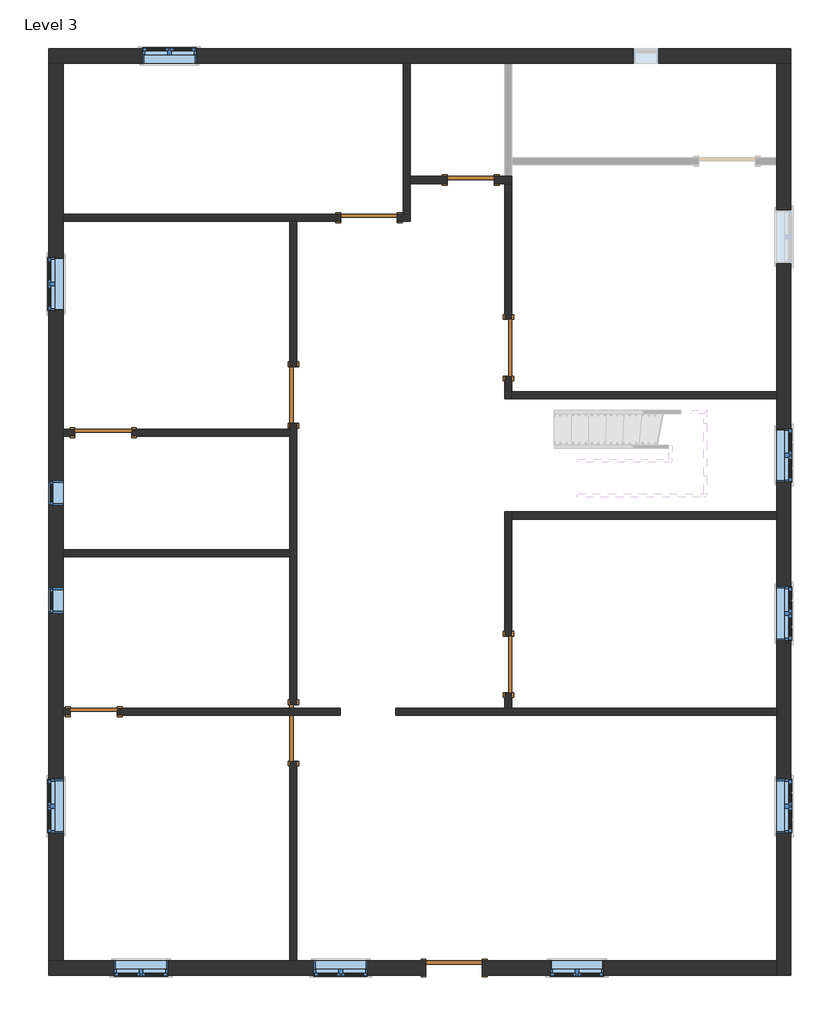
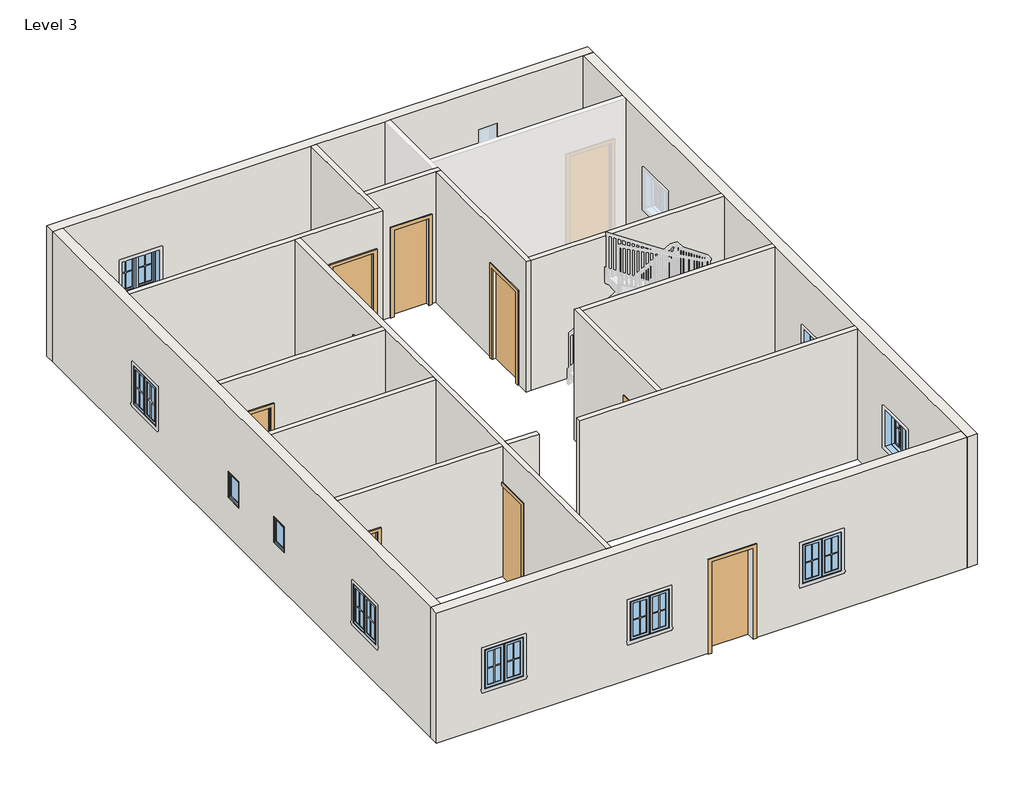
# One storey, part 1 of 3: 16 walls, 11 windows, 9 doors.
"""IFC4 building model written with IfcOpenShell, lengths in millimetres."""

from ifc_helpers import new_model, si_unit, frame, origin, place, context, project, spatial, polyline, outline, extrude, faceted_brep, transform, mapped, element, save
from components import door_d8f5dbb5, door_f2b275c1, door_e5f9f3c4, door_305aa2a5, door_a90ba1ad, window_aa618e30, window_339605e1

model = new_model("IFC4")

# Units and contexts
model_context = context("Model", 3, world=origin())
ifc_project = project(units=[si_unit("LENGTHUNIT", "METRE", prefix="MILLI")], contexts=[model_context])

# Site, building, storey
site = spatial("IfcSite", under=ifc_project)
building = spatial("IfcBuilding", under=site)
storey = spatial("IfcBuildingStorey", under=building, Name="Level 3", Elevation=3200.4)

# Doors
placement = place(None, origin())
door_shape = door_d8f5dbb5(model_context)
element("IfcDoor", 1, ObjectType="Single-Flush : 30\" x 80\"", at=placement, inside=storey, context=model_context, shape_type="MappedRepresentation", body=[
    mapped(door_shape, transform((-509.1743007, 6967.427558, 3200.4), x_axis=(1.0, 0.0, 0.0), y_axis=(0.0, 1.0, 0.0), z_axis=(0.0, 0.0, 1.0))),
])
door_2_shape = door_f2b275c1(model_context)
element("IfcDoor", 2, ObjectType="Single-Flush : 30\" x 80\"", at=placement, inside=storey, context=model_context, shape_type="MappedRepresentation", body=[
    mapped(door_2_shape, transform((-6586.1243007, -1605.072442, 3200.4), x_axis=(-1.0, 0.0, 0.0), y_axis=(0.0, -1.0, 0.0), z_axis=(0.0, 0.0, 1.0))),
])
door_3_shape = door_e5f9f3c4(model_context)
element("IfcDoor", 3, ObjectType="Single-Flush : 36\" x 84\"", at=placement, inside=storey, context=model_context, shape_type="MappedRepresentation", body=[
    mapped(door_3_shape, transform((-2147.4743007, 6357.827558, 3200.4), x_axis=(1.0, 0.0, 0.0), y_axis=(0.0, 1.0, 0.0), z_axis=(0.0, 0.0, 1.0))),
])
element("IfcDoor", 4, ObjectType="Single-Flush : 36\" x 84\"", at=placement, inside=storey, context=model_context, shape_type="MappedRepresentation", body=[
    mapped(door_3_shape, transform((100.4256993, 4262.327558, 3200.4), x_axis=(0.0, -1.0, 0.0), y_axis=(1.0, 0.0, 0.0), z_axis=(0.0, 0.0, 1.0))),
])
element("IfcDoor", 5, ObjectType="Single-Flush : 36\" x 84\"", at=placement, inside=storey, context=model_context, shape_type="MappedRepresentation", body=[
    mapped(door_3_shape, transform((100.4256993, -843.072442, 3200.4), x_axis=(0.0, -1.0, 0.0), y_axis=(1.0, 0.0, 0.0), z_axis=(0.0, 0.0, 1.0))),
])
element("IfcDoor", 6, ObjectType="Single-Flush : 36\" x 84\"", at=placement, inside=storey, context=model_context, shape_type="MappedRepresentation", body=[
    mapped(door_3_shape, transform((-3366.6743007, -1947.972442, 3200.4), x_axis=(0.0, 1.0, 0.0), y_axis=(-1.0, 0.0, 0.0), z_axis=(0.0, 0.0, 1.0))),
])
door_4_shape = door_305aa2a5(model_context)
element("IfcDoor", 7, ObjectType="Single-Flush : 36\" x 84\"", at=placement, inside=storey, context=model_context, shape_type="MappedRepresentation", body=[
    mapped(door_4_shape, transform((-6433.7243007, 2890.727558, 3200.4), x_axis=(-1.0, 0.0, 0.0), y_axis=(0.0, -1.0, 0.0), z_axis=(0.0, 0.0, 1.0))),
])
element("IfcDoor", 8, ObjectType="Single-Flush : 36\" x 84\"", at=placement, inside=storey, context=model_context, shape_type="MappedRepresentation", body=[
    mapped(door_4_shape, transform((-3366.6743007, 3500.327558, 3200.4), x_axis=(0.0, -1.0, 0.0), y_axis=(1.0, 0.0, 0.0), z_axis=(0.0, 0.0, 1.0))),
])
door_5_shape = door_a90ba1ad(model_context)
element("IfcDoor", 9, ObjectType="Single-Flush : 36\" x 84\"", at=placement, inside=storey, context=model_context, shape_type="MappedRepresentation", body=[
    mapped(door_5_shape, transform((-775.8743007, -5738.922442, 3200.4), x_axis=(-1.0, 0.0, 0.0), y_axis=(0.0, -1.0, 0.0), z_axis=(0.0, 0.0, 1.0))),
])

# Walls
element("IfcWall", 10, ObjectType="WALL4.5\"", at=placement, inside=storey, context=model_context, shape_type="Brep", body=[
    faceted_brep([(-1690.2743007, 6300.677558, 5334.0), (-1690.2743007, 6300.677558, 3200.4), (-1480.7243007, 6300.677558, 3200.4), (-1480.7243007, 6300.677558, 6248.4), (-3309.5243007, 6300.677558, 6248.4), (-3423.8243007, 6300.677558, 6248.4), (-7081.4243007, 6300.677558, 6248.4), (-7081.4243007, 6300.677558, 3200.4), (-3423.8243007, 6300.677558, 3200.4), (-3309.5243007, 6300.677558, 3200.4), (-2604.6743007, 6300.677558, 3200.4), (-2604.6743007, 6300.677558, 5334.0), (-1480.7243007, 6414.977558, 3200.4), (-1595.0243007, 6414.977558, 3200.4), (-1690.2743007, 6414.977558, 3200.4), (-1690.2743007, 6414.977558, 5334.0), (-2604.6743007, 6414.977558, 5334.0), (-2604.6743007, 6414.977558, 3200.4), (-7081.4243007, 6414.977558, 3200.4), (-7081.4243007, 6414.977558, 6248.4), (-1595.0243007, 6414.977558, 6248.4), (-1480.7243007, 6414.977558, 6248.4)], [[[0, 1, 2, 3, 4, 5, 6, 7, 8, 9, 10, 11]], [[12, 13, 14, 15, 16, 17, 18, 19, 20, 21]], [[2, 1, 14, 13, 12]], [[10, 9, 8, 7, 18, 17]], [[7, 6, 19, 18]], [[3, 2, 12, 21]], [[15, 14, 1, 0]], [[16, 15, 0, 11]], [[17, 16, 11, 10]], [[6, 5, 4, 3, 21, 20, 19]]]),
])
element("IfcWall", 11, ObjectType="WALL4.5\"", at=placement, inside=storey, context=model_context, shape_type="Brep", body=[
    faceted_brep([(-1480.7243007, 6414.977558, 3200.4), (-1480.7243007, 6910.277558, 3200.4), (-1480.7243007, 7024.577558, 3200.4), (-1480.7243007, 8853.377558, 3200.4), (-1480.7243007, 8853.377558, 6248.4), (-1480.7243007, 7024.577558, 6248.4), (-1480.7243007, 6910.277558, 6248.4), (-1480.7243007, 6414.977558, 6248.4), (-1595.0243007, 6414.977558, 3200.4), (-1595.0243007, 6414.977558, 6248.4), (-1595.0243007, 8853.377558, 6248.4), (-1595.0243007, 8853.377558, 3200.4)], [[[0, 1, 2, 3, 4, 5, 6, 7]], [[8, 9, 10, 11]], [[3, 2, 1, 0, 8, 11]], [[0, 7, 9, 8]], [[4, 3, 11, 10]], [[7, 6, 5, 4, 10, 9]]]),
])
element("IfcWall", 12, ObjectType="WALL4.5\"", at=placement, inside=storey, context=model_context, shape_type="Brep", body=[
    faceted_brep([(-128.1743007, 6910.277558, 5232.4), (-128.1743007, 6910.277558, 3200.4), (43.2756993, 6910.277558, 3200.4), (157.5756993, 6910.277558, 3200.4), (157.5756993, 6910.277558, 6248.4), (43.2756993, 6910.277558, 6248.4), (-1480.7243007, 6910.277558, 6248.4), (-1480.7243007, 6910.277558, 3200.4), (-890.1743007, 6910.277558, 3200.4), (-890.1743007, 6910.277558, 5232.4), (157.5756993, 7024.577558, 3200.4), (43.2756993, 7024.577558, 3200.4), (-128.1743007, 7024.577558, 3200.4), (-128.1743007, 7024.577558, 5232.4), (-890.1743007, 7024.577558, 5232.4), (-890.1743007, 7024.577558, 3200.4), (-1480.7243007, 7024.577558, 3200.4), (-1480.7243007, 7024.577558, 6248.4), (43.2756993, 7024.577558, 6248.4), (157.5756993, 7024.577558, 6248.4)], [[[0, 1, 2, 3, 4, 5, 6, 7, 8, 9]], [[10, 11, 12, 13, 14, 15, 16, 17, 18, 19]], [[8, 7, 16, 15]], [[3, 2, 1, 12, 11, 10]], [[7, 6, 17, 16]], [[4, 3, 10, 19]], [[13, 12, 1, 0]], [[14, 13, 0, 9]], [[15, 14, 9, 8]], [[6, 5, 4, 19, 18, 17]]]),
])
element("IfcWall", 13, ObjectType="WALL4.5\"", at=placement, inside=storey, context=model_context, shape_type="Brep", body=[
    faceted_brep([(-3423.8243007, 3043.127558, 3200.4), (-3423.8243007, 2947.877558, 3200.4), (-3423.8243007, 2833.577558, 3200.4), (-3423.8243007, 1004.777558, 3200.4), (-3423.8243007, 890.477558, 3200.4), (-3423.8243007, -1490.772442, 3200.4), (-3423.8243007, -1490.772442, 5334.0), (-3423.8243007, -1547.922442, 5334.0), (-3423.8243007, -1662.222442, 5334.0), (-3423.8243007, -2405.172442, 5334.0), (-3423.8243007, -2405.172442, 3200.4), (-3423.8243007, -5624.622442, 3200.4), (-3423.8243007, -5624.622442, 6248.4), (-3423.8243007, -1662.222442, 6248.4), (-3423.8243007, -1547.922442, 6248.4), (-3423.8243007, 890.477558, 6248.4), (-3423.8243007, 1004.777558, 6248.4), (-3423.8243007, 2833.577558, 6248.4), (-3423.8243007, 2947.877558, 6248.4), (-3423.8243007, 6300.677558, 6248.4), (-3423.8243007, 6300.677558, 3200.4), (-3423.8243007, 3957.527558, 3200.4), (-3423.8243007, 3957.527558, 5334.0), (-3423.8243007, 3043.127558, 5334.0), (-3309.5243007, -1490.772442, 5334.0), (-3309.5243007, -1490.772442, 3200.4), (-3309.5243007, 3043.127558, 3200.4), (-3309.5243007, 3043.127558, 5334.0), (-3309.5243007, 3957.527558, 5334.0), (-3309.5243007, 3957.527558, 3200.4), (-3309.5243007, 6300.677558, 3200.4), (-3309.5243007, 6300.677558, 6248.4), (-3309.5243007, -1547.922442, 6248.4), (-3309.5243007, -1662.222442, 6248.4), (-3309.5243007, -5624.622442, 6248.4), (-3309.5243007, -5624.622442, 3200.4), (-3309.5243007, -2405.172442, 3200.4), (-3309.5243007, -2405.172442, 5334.0), (-3309.5243007, -1662.222442, 5334.0), (-3309.5243007, -1547.922442, 5334.0)], [[[0, 1, 2, 3, 4, 5, 6, 7, 8, 9, 10, 11, 12, 13, 14, 15, 16, 17, 18, 19, 20, 21, 22, 23]], [[24, 25, 26, 27, 28, 29, 30, 31, 32, 33, 34, 35, 36, 37, 38, 39]], [[21, 20, 30, 29]], [[36, 35, 11, 10]], [[26, 25, 5, 4, 3, 2, 1, 0]], [[12, 11, 35, 34]], [[20, 19, 31, 30]], [[27, 26, 0, 23]], [[28, 27, 23, 22]], [[29, 28, 22, 21]], [[6, 5, 25, 24]], [[9, 8, 7, 6, 24, 39, 38, 37]], [[10, 9, 37, 36]], [[19, 18, 17, 16, 15, 14, 13, 12, 34, 33, 32, 31]]]),
])
element("IfcWall", 14, ObjectType="WALL4.5\"", at=placement, inside=storey, context=model_context, shape_type="Brep", body=[
    faceted_brep([(157.5756993, -1547.922442, 3200.4), (157.5756993, -1300.272442, 3200.4), (157.5756993, -1300.272442, 5334.0), (157.5756993, -385.872442, 5334.0), (157.5756993, -385.872442, 3200.4), (157.5756993, 1500.077558, 3200.4), (157.5756993, 1614.377558, 3200.4), (157.5756993, 1614.377558, 6248.4), (157.5756993, 1500.077558, 6248.4), (157.5756993, -1547.922442, 6248.4), (43.2756993, -1300.272442, 5334.0), (43.2756993, -1300.272442, 3200.4), (43.2756993, -1547.922442, 3200.4), (43.2756993, -1547.922442, 6248.4), (43.2756993, 1614.377558, 6248.4), (43.2756993, 1614.377558, 3200.4), (43.2756993, -385.872442, 3200.4), (43.2756993, -385.872442, 5334.0)], [[[0, 1, 2, 3, 4, 5, 6, 7, 8, 9]], [[10, 11, 12, 13, 14, 15, 16, 17]], [[16, 15, 6, 5, 4]], [[12, 11, 1, 0]], [[7, 6, 15, 14]], [[0, 9, 13, 12]], [[2, 1, 11, 10]], [[3, 2, 10, 17]], [[4, 3, 17, 16]], [[9, 8, 7, 14, 13]]]),
])
element("IfcWall", 15, ObjectType="WALL4.5\"", at=placement, inside=storey, context=model_context, shape_type="SweptSolid", body=[
    extrude(outline(polyline([(4424.7756993, 1500.077558), (157.5756993, 1500.077558), (157.5756993, 1614.377558), (4424.7756993, 1614.377558), (4424.7756993, 1500.077558)])), frame((0.0, 0.0, 3200.4), z_axis=(0.0, 0.0, 1.0), x_axis=(1.0, 0.0, 0.0)), (0.0, 0.0, 1.0), 3048.0),
])
element("IfcWall", 16, ObjectType="WALL4.5\"", at=placement, inside=storey, context=model_context, shape_type="SweptSolid", body=[
    extrude(outline(polyline([(-3423.8243007, 890.477558), (-7081.4243007, 890.477558), (-7081.4243007, 1004.777558), (-3423.8243007, 1004.777558), (-3423.8243007, 890.477558)])), frame((0.0, 0.0, 3200.4), z_axis=(0.0, 0.0, 1.0), x_axis=(1.0, 0.0, 0.0)), (0.0, 0.0, 1.0), 3048.0),
])
element("IfcWall", 17, ObjectType="WALL4.5\"", at=placement, inside=storey, context=model_context, shape_type="SweptSolid", body=[
    extrude(outline(polyline([(3200.4, -7081.4243007), (3200.4, -6890.9243007), (5334.0, -6890.9243007), (5334.0, -5976.5243007), (3200.4, -5976.5243007), (3200.4, -3423.8243007), (6248.4, -3423.8243007), (6248.4, -7081.4243007), (3200.4, -7081.4243007)])), frame((0.0, 2833.577558, 0.0), z_axis=(0.0, 1.0, 0.0), x_axis=(0.0, 0.0, 1.0)), (0.0, 0.0, 1.0), 114.3),
])
element("IfcWall", 18, ObjectType="WALL4.5\"", at=placement, inside=storey, context=model_context, shape_type="Brep", body=[
    faceted_brep([(43.2756993, 3805.127558, 5334.0), (43.2756993, 3805.127558, 3200.4), (43.2756993, 3443.177558, 3200.4), (43.2756993, 3443.177558, 6248.4), (43.2756993, 6910.277558, 6248.4), (43.2756993, 6910.277558, 3200.4), (43.2756993, 4719.527558, 3200.4), (43.2756993, 4719.527558, 5334.0), (157.5756993, 3443.177558, 3200.4), (157.5756993, 3557.477558, 3200.4), (157.5756993, 3805.127558, 3200.4), (157.5756993, 3805.127558, 5334.0), (157.5756993, 4719.527558, 5334.0), (157.5756993, 4719.527558, 3200.4), (157.5756993, 6910.277558, 3200.4), (157.5756993, 6910.277558, 6248.4), (157.5756993, 3557.477558, 6248.4), (157.5756993, 3443.177558, 6248.4)], [[[0, 1, 2, 3, 4, 5, 6, 7]], [[8, 9, 10, 11, 12, 13, 14, 15, 16, 17]], [[6, 5, 14, 13]], [[2, 1, 10, 9, 8]], [[5, 4, 15, 14]], [[3, 2, 8, 17]], [[11, 10, 1, 0]], [[12, 11, 0, 7]], [[13, 12, 7, 6]], [[4, 3, 17, 16, 15]]]),
])
element("IfcWall", 19, ObjectType="WALL4.5\"", at=placement, inside=storey, context=model_context, shape_type="SweptSolid", body=[
    extrude(outline(polyline([(4424.7756993, 3443.177558), (157.5756993, 3443.177558), (157.5756993, 3557.477558), (4424.7756993, 3557.477558), (4424.7756993, 3443.177558)])), frame((0.0, 0.0, 3200.4), z_axis=(0.0, 0.0, 1.0), x_axis=(1.0, 0.0, 0.0)), (0.0, 0.0, 1.0), 3048.0),
])
element("IfcWall", 20, ObjectType="WALL4.5\"", at=placement, inside=storey, context=model_context, shape_type="SweptSolid", body=[
    extrude(outline(polyline([(3200.4, -2614.8628774), (6248.4, -2614.8628774), (6248.4, -3309.5243007), (5334.0, -3309.5243007), (5334.0, -3423.8243007), (6248.4, -3423.8243007), (6248.4, -7081.4243007), (3200.4, -7081.4243007), (3200.4, -6967.1243007), (5232.4, -6967.1243007), (5232.4, -6205.1243007), (3200.4, -6205.1243007), (3200.4, -2614.8628774)])), frame((0.0, -1662.222442, 0.0), z_axis=(0.0, 1.0, 0.0), x_axis=(0.0, 0.0, 1.0)), (0.0, 0.0, 1.0), 114.3),
])
element("IfcWall", 21, ObjectType="WALL4.5\"", at=placement, inside=storey, context=model_context, shape_type="Brep", body=[
    faceted_brep([(-1720.6441625, -1662.222442, 3200.4), (4424.7756993, -1662.222442, 3200.4), (4424.7756993, -1662.222442, 6248.4), (-1720.6441625, -1662.222442, 6248.4), (-1720.6441625, -1547.922442, 3200.4), (-1720.6441625, -1547.922442, 6248.4), (43.2756993, -1547.922442, 6248.4), (157.5756993, -1547.922442, 6248.4), (4424.7756993, -1547.922442, 6248.4), (4424.7756993, -1547.922442, 3200.4), (157.5756993, -1547.922442, 3200.4), (43.2756993, -1547.922442, 3200.4)], [[[0, 1, 2, 3]], [[4, 5, 6, 7, 8, 9, 10, 11]], [[1, 0, 4, 11, 10, 9]], [[0, 3, 5, 4]], [[2, 1, 9, 8]], [[3, 2, 8, 7, 6, 5]]]),
])
element("IfcWall", 22, ObjectType="WALL9\"", at=placement, inside=storey, context=model_context, shape_type="Brep", body=[
    faceted_brep([(-7310.0243007, 8853.377558, 3200.4), (-7081.4243007, 8853.377558, 3200.4), (-1595.0243007, 8853.377558, 3200.4), (-1480.7243007, 8853.377558, 3200.4), (43.2756993, 8853.377558, 3200.4), (157.5756993, 8853.377558, 3200.4), (4424.7756993, 8853.377558, 3200.4), (4653.3756993, 8853.377558, 3200.4), (4653.3756993, 8853.377558, 6248.4), (4424.7756993, 8853.377558, 6248.4), (157.5756993, 8853.377558, 6248.4), (43.2756993, 8853.377558, 6248.4), (-1480.7243007, 8853.377558, 6248.4), (-1595.0243007, 8853.377558, 6248.4), (-7081.4243007, 8853.377558, 6248.4), (-7310.0243007, 8853.377558, 6248.4), (-4935.1243007, 8853.377558, 5029.2), (-4935.1243007, 8853.377558, 4114.8), (-5798.7243007, 8853.377558, 4114.8), (-5798.7243007, 8853.377558, 5029.2), (2522.9506993, 8853.377558, 5334.0), (2522.9506993, 8853.377558, 3505.2), (2116.5506993, 8853.377558, 3505.2), (2116.5506993, 8853.377558, 5334.0), (-7310.0243007, 9081.977558, 3200.4), (-7310.0243007, 9081.977558, 6248.4), (4653.3756993, 9081.977558, 6248.4), (4653.3756993, 9081.977558, 3200.4), (-4935.1243007, 9081.977558, 5029.2), (-5798.7243007, 9081.977558, 5029.2), (-5798.7243007, 9081.977558, 4114.8), (-4935.1243007, 9081.977558, 4114.8), (2522.9506993, 9081.977558, 5334.0), (2116.5506993, 9081.977558, 5334.0), (2116.5506993, 9081.977558, 3505.2), (2522.9506993, 9081.977558, 3505.2)], [[[0, 1, 2, 3, 4, 5, 6, 7, 8, 9, 10, 11, 12, 13, 14, 15], [16, 17, 18, 19], [20, 21, 22, 23]], [[24, 25, 26, 27], [28, 29, 30, 31], [32, 33, 34, 35]], [[7, 6, 5, 4, 3, 2, 1, 0, 24, 27]], [[8, 7, 27, 26]], [[0, 15, 25, 24]], [[17, 16, 28, 31]], [[18, 17, 31, 30]], [[19, 18, 30, 29]], [[16, 19, 29, 28]], [[21, 20, 32, 35]], [[22, 21, 35, 34]], [[23, 22, 34, 33]], [[20, 23, 33, 32]], [[15, 14, 13, 12, 11, 10, 9, 8, 26, 25]]]),
])
element("IfcWall", 23, ObjectType="WALL9\"", at=placement, inside=storey, context=model_context, shape_type="Brep", body=[
    faceted_brep([(4424.7756993, 8853.377558, 3200.4), (4424.7756993, 7329.377558, 3200.4), (4424.7756993, 7215.077558, 3200.4), (4424.7756993, 3557.477558, 3200.4), (4424.7756993, 3443.177558, 3200.4), (4424.7756993, 1614.377558, 3200.4), (4424.7756993, 1500.077558, 3200.4), (4424.7756993, -1547.922442, 3200.4), (4424.7756993, -1662.222442, 3200.4), (4424.7756993, -5624.622442, 3200.4), (4424.7756993, -5853.222442, 3200.4), (4424.7756993, -5853.222442, 6248.4), (4424.7756993, -5624.622442, 6248.4), (4424.7756993, -1662.222442, 6248.4), (4424.7756993, -1547.922442, 6248.4), (4424.7756993, 1500.077558, 6248.4), (4424.7756993, 1614.377558, 6248.4), (4424.7756993, 3443.177558, 6248.4), (4424.7756993, 3557.477558, 6248.4), (4424.7756993, 7215.077558, 6248.4), (4424.7756993, 7329.377558, 6248.4), (4424.7756993, 8853.377558, 6248.4), (4424.7756993, 5621.227558, 5029.2), (4424.7756993, 5621.227558, 4114.8), (4424.7756993, 6484.827558, 4114.8), (4424.7756993, 6484.827558, 5029.2), (4424.7756993, 2096.977558, 5029.2), (4424.7756993, 2096.977558, 4114.8), (4424.7756993, 2960.577558, 4114.8), (4424.7756993, 2960.577558, 5029.2), (4424.7756993, -455.722442, 5029.2), (4424.7756993, -455.722442, 4114.8), (4424.7756993, 407.877558, 4114.8), (4424.7756993, 407.877558, 5029.2), (4424.7756993, -3560.872442, 5029.2), (4424.7756993, -3560.872442, 4114.8), (4424.7756993, -2697.272442, 4114.8), (4424.7756993, -2697.272442, 5029.2), (4653.3756993, 8853.377558, 3200.4), (4653.3756993, 8853.377558, 6248.4), (4653.3756993, -5853.222442, 6248.4), (4653.3756993, -5853.222442, 3200.4), (4653.3756993, 5621.227558, 5029.2), (4653.3756993, 6484.827558, 5029.2), (4653.3756993, 6484.827558, 4114.8), (4653.3756993, 5621.227558, 4114.8), (4653.3756993, 2096.977558, 5029.2), (4653.3756993, 2960.577558, 5029.2), (4653.3756993, 2960.577558, 4114.8), (4653.3756993, 2096.977558, 4114.8), (4653.3756993, -455.722442, 5029.2), (4653.3756993, 407.877558, 5029.2), (4653.3756993, 407.877558, 4114.8), (4653.3756993, -455.722442, 4114.8), (4653.3756993, -3560.872442, 5029.2), (4653.3756993, -2697.272442, 5029.2), (4653.3756993, -2697.272442, 4114.8), (4653.3756993, -3560.872442, 4114.8)], [[[0, 1, 2, 3, 4, 5, 6, 7, 8, 9, 10, 11, 12, 13, 14, 15, 16, 17, 18, 19, 20, 21], [22, 23, 24, 25], [26, 27, 28, 29], [30, 31, 32, 33], [34, 35, 36, 37]], [[38, 39, 40, 41], [42, 43, 44, 45], [46, 47, 48, 49], [50, 51, 52, 53], [54, 55, 56, 57]], [[10, 9, 8, 7, 6, 5, 4, 3, 2, 1, 0, 38, 41]], [[0, 21, 39, 38]], [[11, 10, 41, 40]], [[23, 22, 42, 45]], [[24, 23, 45, 44]], [[25, 24, 44, 43]], [[22, 25, 43, 42]], [[27, 26, 46, 49]], [[28, 27, 49, 48]], [[29, 28, 48, 47]], [[26, 29, 47, 46]], [[31, 30, 50, 53]], [[32, 31, 53, 52]], [[33, 32, 52, 51]], [[30, 33, 51, 50]], [[35, 34, 54, 57]], [[36, 35, 57, 56]], [[37, 36, 56, 55]], [[34, 37, 55, 54]], [[21, 20, 19, 18, 17, 16, 15, 14, 13, 12, 11, 40, 39]]]),
])
element("IfcWall", 24, ObjectType="WALL9\"", at=placement, inside=storey, context=model_context, shape_type="Brep", body=[
    faceted_brep([(-1233.0743007, -5624.622442, 5334.0), (-1233.0743007, -5624.622442, 3200.4), (-3309.5243007, -5624.622442, 3200.4), (-3423.8243007, -5624.622442, 3200.4), (-7081.4243007, -5624.622442, 3200.4), (-7310.0243007, -5624.622442, 3200.4), (-7310.0243007, -5624.622442, 6248.4), (-7081.4243007, -5624.622442, 6248.4), (-3423.8243007, -5624.622442, 6248.4), (-3309.5243007, -5624.622442, 6248.4), (4424.7756993, -5624.622442, 6248.4), (4424.7756993, -5624.622442, 3200.4), (-318.6743007, -5624.622442, 3200.4), (-318.6743007, -5624.622442, 5334.0), (773.5256993, -5624.622442, 5029.2), (773.5256993, -5624.622442, 4114.8), (1637.1256993, -5624.622442, 4114.8), (1637.1256993, -5624.622442, 5029.2), (-3036.4743007, -5624.622442, 5029.2), (-3036.4743007, -5624.622442, 4114.8), (-2172.8743007, -5624.622442, 4114.8), (-2172.8743007, -5624.622442, 5029.2), (-6255.9243007, -5624.622442, 5029.2), (-6255.9243007, -5624.622442, 4114.8), (-5392.3243007, -5624.622442, 4114.8), (-5392.3243007, -5624.622442, 5029.2), (-7310.0243007, -5853.222442, 3200.4), (-1233.0743007, -5853.222442, 3200.4), (-1233.0743007, -5853.222442, 5334.0), (-318.6743007, -5853.222442, 5334.0), (-318.6743007, -5853.222442, 3200.4), (4424.7756993, -5853.222442, 3200.4), (4424.7756993, -5853.222442, 6248.4), (-7310.0243007, -5853.222442, 6248.4), (773.5256993, -5853.222442, 5029.2), (1637.1256993, -5853.222442, 5029.2), (1637.1256993, -5853.222442, 4114.8), (773.5256993, -5853.222442, 4114.8), (-3036.4743007, -5853.222442, 5029.2), (-2172.8743007, -5853.222442, 5029.2), (-2172.8743007, -5853.222442, 4114.8), (-3036.4743007, -5853.222442, 4114.8), (-6255.9243007, -5853.222442, 5029.2), (-5392.3243007, -5853.222442, 5029.2), (-5392.3243007, -5853.222442, 4114.8), (-6255.9243007, -5853.222442, 4114.8)], [[[0, 1, 2, 3, 4, 5, 6, 7, 8, 9, 10, 11, 12, 13], [14, 15, 16, 17], [18, 19, 20, 21], [22, 23, 24, 25]], [[26, 27, 28, 29, 30, 31, 32, 33], [34, 35, 36, 37], [38, 39, 40, 41], [42, 43, 44, 45]], [[12, 11, 31, 30]], [[5, 4, 3, 2, 1, 27, 26]], [[11, 10, 32, 31]], [[6, 5, 26, 33]], [[28, 27, 1, 0]], [[29, 28, 0, 13]], [[30, 29, 13, 12]], [[15, 14, 34, 37]], [[16, 15, 37, 36]], [[17, 16, 36, 35]], [[14, 17, 35, 34]], [[19, 18, 38, 41]], [[20, 19, 41, 40]], [[21, 20, 40, 39]], [[18, 21, 39, 38]], [[23, 22, 42, 45]], [[24, 23, 45, 44]], [[25, 24, 44, 43]], [[22, 25, 43, 42]], [[10, 9, 8, 7, 6, 33, 32]]]),
])
element("IfcWall", 25, ObjectType="WALL9\"", at=placement, inside=storey, context=model_context, shape_type="Brep", body=[
    faceted_brep([(-7081.4243007, -5624.622442, 3200.4), (-7081.4243007, -1662.222442, 3200.4), (-7081.4243007, -1547.922442, 3200.4), (-7081.4243007, 890.477558, 3200.4), (-7081.4243007, 1004.777558, 3200.4), (-7081.4243007, 2833.577558, 3200.4), (-7081.4243007, 2947.877558, 3200.4), (-7081.4243007, 6300.677558, 3200.4), (-7081.4243007, 6414.977558, 3200.4), (-7081.4243007, 8853.377558, 3200.4), (-7081.4243007, 8853.377558, 6248.4), (-7081.4243007, 6414.977558, 6248.4), (-7081.4243007, 6300.677558, 6248.4), (-7081.4243007, 2947.877558, 6248.4), (-7081.4243007, 2833.577558, 6248.4), (-7081.4243007, 1004.777558, 6248.4), (-7081.4243007, 890.477558, 6248.4), (-7081.4243007, -1547.922442, 6248.4), (-7081.4243007, -1662.222442, 6248.4), (-7081.4243007, -5624.622442, 6248.4), (-7081.4243007, 388.827558, 4724.4), (-7081.4243007, 388.827558, 4114.8), (-7081.4243007, -17.572442, 4114.8), (-7081.4243007, -17.572442, 4724.4), (-7081.4243007, 2122.377558, 4724.4), (-7081.4243007, 2122.377558, 4114.8), (-7081.4243007, 1715.977558, 4114.8), (-7081.4243007, 1715.977558, 4724.4), (-7081.4243007, 5722.827558, 5029.2), (-7081.4243007, 5722.827558, 4114.8), (-7081.4243007, 4859.227558, 4114.8), (-7081.4243007, 4859.227558, 5029.2), (-7081.4243007, -2697.272442, 5029.2), (-7081.4243007, -2697.272442, 4114.8), (-7081.4243007, -3560.872442, 4114.8), (-7081.4243007, -3560.872442, 5029.2), (-7310.0243007, -5624.622442, 3200.4), (-7310.0243007, -5624.622442, 6248.4), (-7310.0243007, 8853.377558, 6248.4), (-7310.0243007, 8853.377558, 3200.4), (-7310.0243007, 388.827558, 4724.4), (-7310.0243007, -17.572442, 4724.4), (-7310.0243007, -17.572442, 4114.8), (-7310.0243007, 388.827558, 4114.8), (-7310.0243007, 2122.377558, 4724.4), (-7310.0243007, 1715.977558, 4724.4), (-7310.0243007, 1715.977558, 4114.8), (-7310.0243007, 2122.377558, 4114.8), (-7310.0243007, 5722.827558, 5029.2), (-7310.0243007, 4859.227558, 5029.2), (-7310.0243007, 4859.227558, 4114.8), (-7310.0243007, 5722.827558, 4114.8), (-7310.0243007, -2697.272442, 5029.2), (-7310.0243007, -3560.872442, 5029.2), (-7310.0243007, -3560.872442, 4114.8), (-7310.0243007, -2697.272442, 4114.8)], [[[0, 1, 2, 3, 4, 5, 6, 7, 8, 9, 10, 11, 12, 13, 14, 15, 16, 17, 18, 19], [20, 21, 22, 23], [24, 25, 26, 27], [28, 29, 30, 31], [32, 33, 34, 35]], [[36, 37, 38, 39], [40, 41, 42, 43], [44, 45, 46, 47], [48, 49, 50, 51], [52, 53, 54, 55]], [[9, 8, 7, 6, 5, 4, 3, 2, 1, 0, 36, 39]], [[10, 9, 39, 38]], [[0, 19, 37, 36]], [[21, 20, 40, 43]], [[22, 21, 43, 42]], [[23, 22, 42, 41]], [[20, 23, 41, 40]], [[25, 24, 44, 47]], [[26, 25, 47, 46]], [[27, 26, 46, 45]], [[24, 27, 45, 44]], [[29, 28, 48, 51]], [[30, 29, 51, 50]], [[31, 30, 50, 49]], [[28, 31, 49, 48]], [[33, 32, 52, 55]], [[34, 33, 55, 54]], [[35, 34, 54, 53]], [[32, 35, 53, 52]], [[19, 18, 17, 16, 15, 14, 13, 12, 11, 10, 38, 37]]]),
])

# Windows
window_shape = window_aa618e30(model_context)
element("IfcWindow", 26, ObjectType="Fixed : 16\" x 24\"", at=placement, inside=storey, context=model_context, shape_type="MappedRepresentation", body=[
    mapped(window_shape, transform((-7195.7243007, 223.727558, 3200.4), x_axis=(0.0, 1.0, 0.0), y_axis=(-1.0, 0.0, 0.0), z_axis=(0.0, 0.0, 1.0))),
])
element("IfcWindow", 27, ObjectType="Fixed : 16\" x 24\"", at=placement, inside=storey, context=model_context, shape_type="MappedRepresentation", body=[
    mapped(window_shape, transform((-7195.7243007, 1957.277558, 3200.4), x_axis=(0.0, 1.0, 0.0), y_axis=(-1.0, 0.0, 0.0), z_axis=(0.0, 0.0, 1.0))),
])
window_2_shape = window_339605e1(model_context)
element("IfcWindow", 28, ObjectType="Window-Casement-Double : 34\" x 36\"", at=placement, inside=storey, context=model_context, shape_type="MappedRepresentation", body=[
    mapped(window_2_shape, transform((-5366.9243007, 8967.677558, 3200.4), x_axis=(1.0, 0.0, 0.0), y_axis=(0.0, 1.0, 0.0), z_axis=(0.0, 0.0, 1.0))),
])
element("IfcWindow", 29, ObjectType="Window-Casement-Double : 34\" x 36\"", at=placement, inside=storey, context=model_context, shape_type="MappedRepresentation", body=[
    mapped(window_2_shape, transform((-7195.7243007, 5291.027558, 3200.4), x_axis=(0.0, 1.0, 0.0), y_axis=(-1.0, 0.0, 0.0), z_axis=(0.0, 0.0, 1.0))),
])
element("IfcWindow", 30, ObjectType="Window-Casement-Double : 34\" x 36\"", at=placement, inside=storey, context=model_context, shape_type="MappedRepresentation", body=[
    mapped(window_2_shape, transform((4539.0756993, 2528.777558, 3200.4), x_axis=(0.0, -1.0, 0.0), y_axis=(1.0, 0.0, 0.0), z_axis=(0.0, 0.0, 1.0))),
])
element("IfcWindow", 31, ObjectType="Window-Casement-Double : 34\" x 36\"", at=placement, inside=storey, context=model_context, shape_type="MappedRepresentation", body=[
    mapped(window_2_shape, transform((4539.0756993, -23.922442, 3200.4), x_axis=(0.0, -1.0, 0.0), y_axis=(1.0, 0.0, 0.0), z_axis=(0.0, 0.0, 1.0))),
])
element("IfcWindow", 32, ObjectType="Window-Casement-Double : 34\" x 36\"", at=placement, inside=storey, context=model_context, shape_type="MappedRepresentation", body=[
    mapped(window_2_shape, transform((4539.0756993, -3129.072442, 3200.4), x_axis=(0.0, -1.0, 0.0), y_axis=(1.0, 0.0, 0.0), z_axis=(0.0, 0.0, 1.0))),
])
element("IfcWindow", 33, ObjectType="Window-Casement-Double : 34\" x 36\"", at=placement, inside=storey, context=model_context, shape_type="MappedRepresentation", body=[
    mapped(window_2_shape, transform((1205.3256993, -5738.922442, 3200.4), x_axis=(-1.0, 0.0, 0.0), y_axis=(0.0, -1.0, 0.0), z_axis=(0.0, 0.0, 1.0))),
])
element("IfcWindow", 34, ObjectType="Window-Casement-Double : 34\" x 36\"", at=placement, inside=storey, context=model_context, shape_type="MappedRepresentation", body=[
    mapped(window_2_shape, transform((-2604.6743007, -5738.922442, 3200.4), x_axis=(-1.0, 0.0, 0.0), y_axis=(0.0, -1.0, 0.0), z_axis=(0.0, 0.0, 1.0))),
])
element("IfcWindow", 35, ObjectType="Window-Casement-Double : 34\" x 36\"", at=placement, inside=storey, context=model_context, shape_type="MappedRepresentation", body=[
    mapped(window_2_shape, transform((-5824.1243007, -5738.922442, 3200.4), x_axis=(-1.0, 0.0, 0.0), y_axis=(0.0, -1.0, 0.0), z_axis=(0.0, 0.0, 1.0))),
])
element("IfcWindow", 36, ObjectType="Window-Casement-Double : 34\" x 36\"", at=placement, inside=storey, context=model_context, shape_type="MappedRepresentation", body=[
    mapped(window_2_shape, transform((-7195.7243007, -3129.072442, 3200.4), x_axis=(0.0, 1.0, 0.0), y_axis=(-1.0, 0.0, 0.0), z_axis=(0.0, 0.0, 1.0))),
])

save(model, "model.ifc")

# Revit data of these elements
# Type "Single-Flush : 30\" x 80\""
#   Type Mark = "5"
#   Construction Type Id = "MDOOR"
#   Assembly Code = "C1020"
#   Analytic Construction = "Metal"
#   Thickness = 0' - 2"
#   Heat Transfer Coefficient (U) = 0.651978 BTU/(h·ft²·°F)
#   Height = 6' - 8"
#   Trim Projection Ext = 0' - 1"
#   Trim Projection Int = 0' - 1"
#   Trim Width = 0' - 3"
#   Width = 2' - 6"
#   Define Thermal Properties by = 1
#   Define Thermal Properties by = 1
#   Door Material = Door - Panel
#   Frame Material = Door - Frame
#   Visual Light Transmittance = 0
#   Solar Heat Gain Coefficient = 0
#   Function = (empty or 0)
#   Wall Closure = (empty or 0)
# Type "Single-Flush : 36\" x 84\""
#   Type Mark = "1"
#   Construction Type Id = "MDOOR"
#   Assembly Code = "C1020"
#   Analytic Construction = "Metal"
#   Thickness = 0' - 2"
#   Heat Transfer Coefficient (U) = 0.651978 BTU/(h·ft²·°F)
#   Height = 7' - 0"
#   Trim Projection Ext = 0' - 1"
#   Trim Projection Int = 0' - 1"
#   Trim Width = 0' - 3"
#   Width = 3' - 0"
#   Define Thermal Properties by = 1
#   Define Thermal Properties by = 1
#   Door Material = Door - Panel
#   Frame Material = Door - Frame
#   Visual Light Transmittance = 0
#   Solar Heat Gain Coefficient = 0
#   Function = (empty or 0)
#   Wall Closure = (empty or 0)
# Type "WALL4.5\""
#   Assembly Code = "B2010"
#   Layers, outside or top first: 0' - 4 1/2" no material (function 1)
# Type "WALL9\""
#   Assembly Code = "B2010"
#   Layers, outside or top first: 0' - 9" no material (function 1)
# Type "Fixed : 16\" x 24\""
#   Type Mark = "4"
#   Construction Type Id = "GSP4R"
#   Assembly Code = "B2020100"
#   Analytic Construction = "1/8 in Pilkington single glazing"
#   Visual Light Transmittance = 0.9
#   Solar Heat Gain Coefficient = 0.78
#   Heat Transfer Coefficient (U) = 0.6496 BTU/(h·ft²·°F)
#   Height = 2' - 0"
#   Default Sill Height = 3' - 0"
#   Width = 1' - 4"
#   Window Inset = 0' - 0 3/4"
#   Define Thermal Properties by = 1
#   Define Thermal Properties by = 1
#   Glass Pane Material = Glass
#   Sash Material = Sash
#   Wall Closure = (empty or 0)
# Type "Window-Casement-Double : 34\" x 36\""
#   Type Mark = "14"
#   Fire Rating = "0.5h"
#   Assembly Code = "B2020100"
#   Analytic Construction = "Double glazing - domestic"
#   Frame Extension [instance default] = 0' - 0 1/4"
#   Window Inset [instance default] = 0' - 0"
#   Wall Thickness [instance default] = 0' - 6"
#   Interior Wall Closure [instance default] = 0' - 2 1/4"
#   Half Width = 1' - 5"
#   Visual Light Transmittance = 0.81
#   Thermal Resistance (R) = 1.8146 (h·ft²·°F)/BTU
#   Solar Heat Gain Coefficient = 0.76
#   Rough Width = 2' - 10 1/2"
#   Rough Height = 3' - 0 1/2"
#   Height = 3' - 0"
#   Heat Transfer Coefficient (U) = 0.5511 BTU/(h·ft²·°F)
#   Exterior Wall Closure [instance default] = 0' - 1 1/4"
#   Extension Jamb [instance default] = 0' - 2 1/4"
#   Default Sill Height = 3' - 0"
#   Width = 2' - 10"
#   Define Thermal Properties by = 0
#   Muntin Visibility = yes
#   Interior Trim Visibility [instance default] = yes
#   Exterior Trim Visibility [instance default] = yes
#   Extension Jamb Visibility [instance default] = yes
#   Interior Trim Material = Wood - Stained
#   Muntin Pattern = Muntin Pattern_2x2 : Muntin Pattern_2x2
#   Interior Trim = Trim-Window-Interior-Flat : Picture Frame
#   Interior Frame Material = Wood - Stained
#   Glass Panel Material = Glass
#   Exterior Trim Material = Clad - White
#   Exterior Trim = Trim-Window-Exterior-Flat : with Sill
#   Exterior Frame Material = Clad - White
#   Wall Closure = (empty or 0)
# Elements 1, 2 (IfcDoor, "Single-Flush : 30\" x 80\"")
#   Phase Created = New Construction
#   Materials on its faces: "Door - Frame", "Door - Panel"
# Elements 3, 4, 5, 6, 7, 8, 9 (IfcDoor, "Single-Flush : 36\" x 84\"")
#   Phase Created = New Construction
#   Materials on its faces: "Door - Frame", "Door - Panel"
# Elements 10, 11, 12, 13, 14, 15, 16, 17, 18, 19, 20, 21 (IfcWall, "WALL4.5\"")
#   Top Offset = 0' - 0"
#   Base Offset = 0' - 0"
#   Unconnected Height = 10' - 0"
#   wall height = 10' - 0"
#   Phase Created = New Construction
#   Base Constraint = Level 3
#   Materials on its faces: "Default Wall"
# Elements 22, 23, 24, 25 (IfcWall, "WALL9\"")
#   Top Offset = 0' - 0"
#   Base Offset = 0' - 0"
#   Unconnected Height = 10' - 0"
#   wall height = 10' - 0"
#   Phase Created = New Construction
#   Base Constraint = Level 3
#   Materials on its faces: "Default Wall"
# Element 26 (IfcWindow, "Fixed : 16\" x 24\"")
#   Mark = "15"
#   Phase Created = New Construction
#   Materials on its faces: "Sash", "Glass"
# Element 27 (IfcWindow, "Fixed : 16\" x 24\"")
#   Mark = "17"
#   Phase Created = New Construction
#   Materials on its faces: "Sash", "Glass"
# Element 28 (IfcWindow, "Window-Casement-Double : 34\" x 36\"")
#   Mark = "16"
#   Window Inset = 0' - 0"
#   Interior Wall Closure = 0' - 2 1/4"
#   Frame Extension = 0' - 0 1/4"
#   Exterior Wall Closure = 0' - 1 1/4"
#   Interior Trim Visibility = yes
#   Exterior Trim Visibility = yes
#   Phase Created = New Construction
#   Materials on its faces: "Wood - Stained", "Glass", "Clad - White"
# Element 29 (IfcWindow, "Window-Casement-Double : 34\" x 36\"")
#   Mark = "18"
#   Window Inset = 0' - 0"
#   Interior Wall Closure = 0' - 2 1/4"
#   Frame Extension = 0' - 0 1/4"
#   Exterior Wall Closure = 0' - 1 1/4"
#   Interior Trim Visibility = yes
#   Exterior Trim Visibility = yes
#   Phase Created = New Construction
#   Materials on its faces: "Wood - Stained", "Glass", "Clad - White"
# Element 30 (IfcWindow, "Window-Casement-Double : 34\" x 36\"")
#   Mark = "20"
#   Window Inset = 0' - 0"
#   Interior Wall Closure = 0' - 2 1/4"
#   Frame Extension = 0' - 0 1/4"
#   Exterior Wall Closure = 0' - 1 1/4"
#   Interior Trim Visibility = yes
#   Exterior Trim Visibility = yes
#   Phase Created = New Construction
#   Materials on its faces: "Wood - Stained", "Glass", "Clad - White"
# Element 31 (IfcWindow, "Window-Casement-Double : 34\" x 36\"")
#   Mark = "21"
#   Window Inset = 0' - 0"
#   Interior Wall Closure = 0' - 2 1/4"
#   Frame Extension = 0' - 0 1/4"
#   Exterior Wall Closure = 0' - 1 1/4"
#   Interior Trim Visibility = yes
#   Exterior Trim Visibility = yes
#   Phase Created = New Construction
#   Materials on its faces: "Wood - Stained", "Glass", "Clad - White"
# Element 32 (IfcWindow, "Window-Casement-Double : 34\" x 36\"")
#   Mark = "22"
#   Window Inset = 0' - 0"
#   Interior Wall Closure = 0' - 2 1/4"
#   Frame Extension = 0' - 0 1/4"
#   Exterior Wall Closure = 0' - 1 1/4"
#   Interior Trim Visibility = yes
#   Exterior Trim Visibility = yes
#   Phase Created = New Construction
#   Materials on its faces: "Wood - Stained", "Glass", "Clad - White"
# Element 33 (IfcWindow, "Window-Casement-Double : 34\" x 36\"")
#   Mark = "23"
#   Window Inset = 0' - 0"
#   Interior Wall Closure = 0' - 2 1/4"
#   Frame Extension = 0' - 0 1/4"
#   Exterior Wall Closure = 0' - 1 1/4"
#   Interior Trim Visibility = yes
#   Exterior Trim Visibility = yes
#   Phase Created = New Construction
#   Materials on its faces: "Wood - Stained", "Glass", "Clad - White"
# Element 34 (IfcWindow, "Window-Casement-Double : 34\" x 36\"")
#   Mark = "24"
#   Window Inset = 0' - 0"
#   Interior Wall Closure = 0' - 2 1/4"
#   Frame Extension = 0' - 0 1/4"
#   Exterior Wall Closure = 0' - 1 1/4"
#   Interior Trim Visibility = yes
#   Exterior Trim Visibility = yes
#   Phase Created = New Construction
#   Materials on its faces: "Wood - Stained", "Glass", "Clad - White"
# Element 35 (IfcWindow, "Window-Casement-Double : 34\" x 36\"")
#   Mark = "25"
#   Window Inset = 0' - 0"
#   Interior Wall Closure = 0' - 2 1/4"
#   Frame Extension = 0' - 0 1/4"
#   Exterior Wall Closure = 0' - 1 1/4"
#   Interior Trim Visibility = yes
#   Exterior Trim Visibility = yes
#   Phase Created = New Construction
#   Materials on its faces: "Wood - Stained", "Glass", "Clad - White"
# Element 36 (IfcWindow, "Window-Casement-Double : 34\" x 36\"")
#   Mark = "26"
#   Window Inset = 0' - 0"
#   Interior Wall Closure = 0' - 2 1/4"
#   Frame Extension = 0' - 0 1/4"
#   Exterior Wall Closure = 0' - 1 1/4"
#   Interior Trim Visibility = yes
#   Exterior Trim Visibility = yes
#   Phase Created = New Construction
#   Materials on its faces: "Wood - Stained", "Glass", "Clad - White"
# Materials
#   "Door - Panel": class "Wood", colour RGB 210 159 95, transparency 0, Cost = 0
#   "Door - Frame": colour RGB 118 70 51, transparency 0, Cost = 0
#   "Glass": class "Glass", colour RGB 0 128 192, transparency 0.75, Description = "Soda Lime Glass", Cost = 0
#   "Sash": class "Wood", colour RGB 224 178 126, transparency 0, Cost = 0
#   "Wood - Stained": class "Wood", colour RGB 224 178 126, transparency 0, Cost = 0
#   "Clad - White": class "Wood", colour RGB 242 242 238, transparency 0, Cost = 0
#   "Default Wall": colour RGB 128 128 128, transparency 0, Cost = 0
